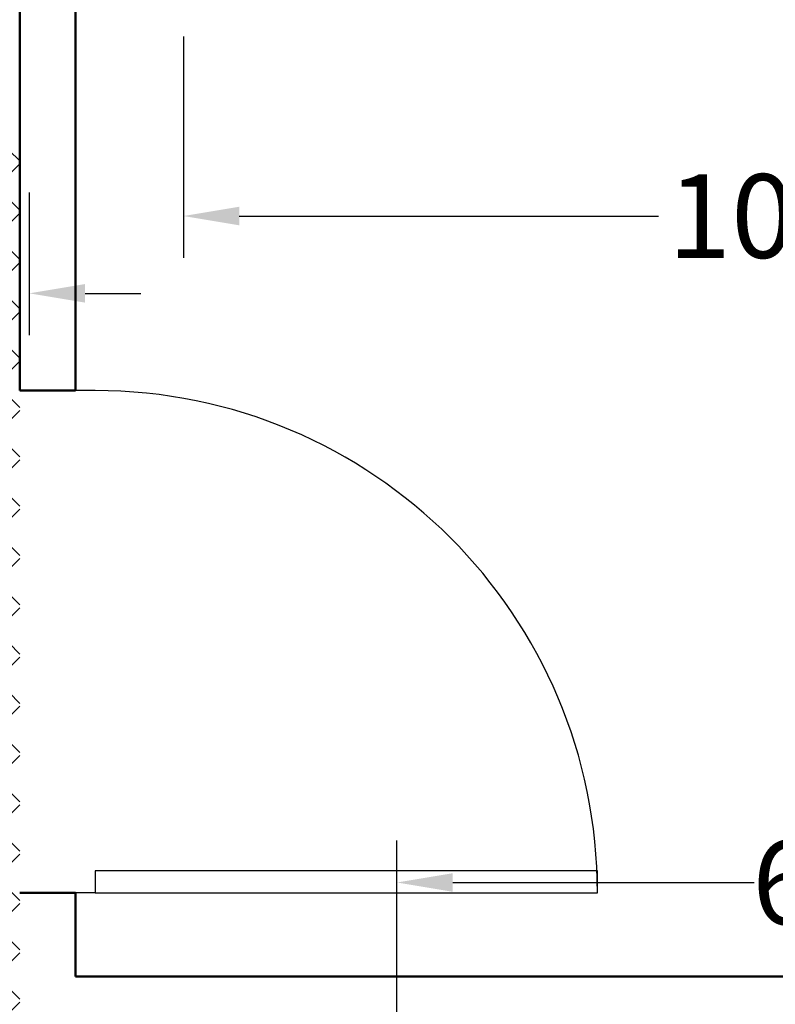
# Model space of a CAD drawing. Units: inches. Extents: x -466983 to 1020, y 324 to 318697.
# Tile 93 of 97: x 810 to 864, y 827 to 898. Entities that reach past the tile are written whole.
import ezdxf

# ---------------------------------------------------------------- set-up
doc = ezdxf.new("R2010")
doc.units = ezdxf.units.IN
doc.header["$MEASUREMENT"] = 0
for name, color, linetype, lineweight in [('A-ANNO-DIMS', 2, 'Continuous', 18), ('A-DOOR', 3, 'Continuous', 25), ('A-FLOR-PATT', 252, 'Continuous', 13), ('A-FURN', 8, 'Continuous', 18), ('A-WALL', 7, 'Continuous', 50)]:
    doc.layers.add(name, color=color, linetype=linetype, lineweight=lineweight)
doc.styles.get("Standard").update_dxf_attribs({"font": 'arial.ttf'})
doc.dimstyles.get("Standard").update_dxf_attribs({"dimtxt": 6, "dimasz": 4, "dimexe": 3, "dimexo": 3, "dimgap": 0.09, "dimtad": 0, "dimtih": 1, "dimtoh": 1, "dimdec": 1, "dimzin": 0, "dimdsep": 46, "dimlunit": 3, "dimtxsty": 'Standard', "dimcen": 0.09, "dimadec": 0, "dimazin": 0, "dimtfac": 1, "dimtdec": 1, "dimtofl": 0, "dimtmove": 0, "dimatfit": 3, "dimfxl": 1, "dimtolj": 1, "dimtzin": 0, "dimarcsym": 0})

# ---------------------------------------------------------------- blocks, each defined once
blk = doc.blocks.new('*U36')
for p, q in [((0, 0), (0, 6)), ((40, 0), (40, 6))]:
    blk.add_line(p, q)
blk.add_lwpolyline([(0, 0), (0, -40), (1.75, -40), (1.75, 0)], close=True)
blk.add_arc((0, 0), 40, 270, 0)
blk = doc.blocks.new('L Shaped Sofa')
at = {"ltscale": 2}
blk.add_arc((2416.36, 1205.03), 481.82, 262.8867, 276.632, dxfattribs=at)
blk = doc.blocks.new('*D71')
at = {"layer": 'A-ANNO-DIMS', "color": 0, "lineweight": -2, "transparency": 16777216}
for p, q in [((742.215, 885.152), (742.215, 874.91)), ((810.492, 885.152), (810.492, 874.91)), ((738.215, 877.91), (734.215, 877.91)), ((814.492, 877.91), (818.492, 877.91))]:
    blk.add_line(p, q, dxfattribs=at)
at = {"layer": 'A-ANNO-DIMS', "color": 0, "transparency": 16777216}
for points in [[(738.215, 878.577), (738.215, 877.244), (742.215, 877.91)], [(814.492, 878.577), (814.492, 877.244), (810.492, 877.91)]]:
    blk.add_solid(points, dxfattribs=at)
at = {"layer": 'Defpoints', "color": 0, "transparency": 16777216}
for p in [(742.215, 888.152), (810.492, 888.152), (742.215, 877.91)]:
    blk.add_point(p, dxfattribs=at)
at = {"layer": 'A-ANNO-DIMS', "color": 0, "transparency": 16777216, "insert": (776.354, 877.91), "char_height": 6, "attachment_point": 5}
blk.add_mtext('\\A1;L-SOFA 68 TYP.', dxfattribs=at)
blk = doc.blocks.new('*D74')
at = {"layer": 'A-ANNO-DIMS', "color": 0, "lineweight": -2, "transparency": 16777216}
for p, q in [((821.534, 896.315), (821.534, 880.453)), ((923.134, 896.315), (923.134, 880.453)), ((825.534, 883.453), (855.592, 883.453)), ((919.134, 883.453), (889.075, 883.453))]:
    blk.add_line(p, q, dxfattribs=at)
at = {"layer": 'A-ANNO-DIMS', "color": 0, "transparency": 16777216}
for points in [[(825.534, 884.119), (825.534, 882.786), (821.534, 883.453)], [(919.134, 884.119), (919.134, 882.786), (923.134, 883.453)]]:
    blk.add_solid(points, dxfattribs=at)
at = {"layer": 'Defpoints', "color": 0, "transparency": 16777216}
for p in [(821.534, 899.315), (923.134, 899.315), (923.134, 883.453)]:
    blk.add_point(p, dxfattribs=at)
at = {"layer": 'A-ANNO-DIMS', "color": 0, "transparency": 16777216, "insert": (872.334, 883.453), "char_height": 6, "attachment_point": 5}
blk.add_mtext('\\A1;102 TYP.', dxfattribs=at)
blk = doc.blocks.new('*D100')
at = {"layer": 'A-ANNO-DIMS', "color": 0, "lineweight": -2, "transparency": 16777216}
for p, q in [((836.84, 825.679), (836.84, 838.67)), ((896.84, 825.679), (896.84, 838.67)), ((840.84, 835.67), (862.447, 835.67)), ((892.84, 835.67), (871.234, 835.67))]:
    blk.add_line(p, q, dxfattribs=at)
at = {"layer": 'A-ANNO-DIMS', "color": 0, "transparency": 16777216}
for points in [[(840.84, 836.336), (840.84, 835.003), (836.84, 835.67)], [(892.84, 836.336), (892.84, 835.003), (896.84, 835.67)]]:
    blk.add_solid(points, dxfattribs=at)
at = {"layer": 'Defpoints', "color": 0, "transparency": 16777216}
for p in [(896.84, 835.67), (836.84, 822.679), (896.84, 822.679)]:
    blk.add_point(p, dxfattribs=at)
at = {"layer": 'A-ANNO-DIMS', "color": 0, "transparency": 16777216, "insert": (866.84, 835.67), "char_height": 6, "attachment_point": 5}
blk.add_mtext('\\A1;60', dxfattribs=at)

msp = doc.modelspace()

# ---------------------------------------------------------------- hatches: boundary and pattern name
at = {"layer": 'A-FLOR-PATT', "transparency": 33554572}
h = msp.add_hatch(dxfattribs=at)
h.set_pattern_fill('ANSI37', color=256, scale=30)
h.set_pattern_definition([(45, (-1212.4137, -290.035), (-2.6516504, 2.6516504), []), (135, (-1212.4137, -290.035), (-2.6516504, -2.6516504), [])])
h.paths.add_polyline_path([(901.806, 1075.938), (900.614, 1075.938), (900.614, 1065.386), (899.391, 1065.386), (898.091, 1065.386), (892.836, 1058.71, -0.258377), (892.188, 1058.351), (879.985, 1058.351, -0.20177), (879.438, 1058.581), (874.081, 1065.386), (872.781, 1065.386), (871.558, 1065.386), (871.558, 1075.938), (813.806, 1075.938), (813.806, 1044.792), (832.395, 1044.792, -0.394795), (848.66, 1028.536), (848.66, 1009.938), (901.806, 1009.938), (901.806, 1015.938), (901.306, 1015.938), (871.306, 1015.938), (871.306, 1017.25), (871.334, 1017.25, -0.401453), (901.306, 1045.938), (901.806, 1045.938)])
edge = h.paths.add_edge_path(flags=16)
edge.add_line((847.773, 1068.949), (847.773, 1073.709))
edge.add_arc((849.227, 1073.709), 1.454, 90, 180, ccw=False)
edge.add_line((849.227, 1075.163), (864.492, 1075.163))
edge.add_arc((864.492, 1073.709), 1.454, 0, 90, ccw=False)
edge.add_line((865.946, 1073.709), (865.946, 1069.004))
edge.add_arc((832.645, 1068.976), 33.301, -20.61234, 0.04725, ccw=False)
edge.add_ellipse((856.859, 1058.48), major_axis=(0, 10.213), ratio=0.685919, start_angle=100.00884, end_angle=259.99116, ccw=False)
edge.add_arc((881.074, 1068.976), 33.301, 180.04725, 200.61234, ccw=False)
h.paths.add_polyline_path([(853.146, 1066.482), (853.146, 1066.453), (853.146, 1066.453, 0.433107), (852.917, 1066.685), (852.917, 1066.453), (853.146, 1066.453), (853.146, 1066.482), (853.088, 1066.612, 0.697939), (852.7, 1066.453), (852.7, 1066.453), (852.7, 1066.482), (852.917, 1067.001), (852.917, 1066.685, -0.396254)], flags=0)
h.paths.add_polyline_path([(861.019, 1066.482), (861.019, 1066.453), (861.019, 1066.453, 0.416404), (860.802, 1066.685), (860.802, 1066.453), (861.019, 1066.453), (861.019, 1066.482), (860.967, 1066.605, 0.713344), (860.573, 1066.453), (860.573, 1066.453), (860.573, 1066.482), (860.802, 1067.001), (860.802, 1066.685, -0.379973)], flags=0)
edge = h.paths.add_edge_path(flags=0)
edge.add_spline(control_points=[(861.13, 1065.785), (861.466, 1065.248), (861.613, 1065.016), (861.983, 1064.374), (862.192, 1063.944), (862.561, 1063.039), (862.721, 1062.563), (862.987, 1061.578), (863.092, 1061.069), (863.245, 1060.031), (863.293, 1059.503), (863.329, 1058.441), (863.318, 1057.908), (863.237, 1056.852), (863.166, 1056.329), (862.97, 1055.308), (862.843, 1054.81), (862.537, 1053.852), (862.357, 1053.393), (861.951, 1052.525), (861.725, 1052.117), (861.233, 1051.362), (860.967, 1051.016), (860.405, 1050.395), (860.108, 1050.12), (859.494, 1049.646), (859.176, 1049.448), (858.528, 1049.13), (858.197, 1049.011), (857.531, 1048.852), (857.196, 1048.812), (856.525, 1048.812), (856.189, 1048.852), (855.524, 1049.01), (855.193, 1049.129), (854.545, 1049.447), (854.227, 1049.645), (853.612, 1050.118), (853.316, 1050.393), (852.753, 1051.014), (852.487, 1051.36), (851.995, 1052.114), (851.769, 1052.523), (851.363, 1053.39), (851.183, 1053.85), (850.877, 1054.807), (850.75, 1055.305), (850.553, 1056.326), (850.483, 1056.849), (850.401, 1057.905), (850.39, 1058.438), (850.426, 1059.5), (850.473, 1060.028), (850.626, 1061.066), (850.732, 1061.575), (850.997, 1062.561), (851.157, 1063.036), (851.525, 1063.942), (851.734, 1064.371), (852.106, 1065.016), (852.254, 1065.25), (852.608, 1065.733)], knot_values=[3.915332, 3.915332, 3.915332, 3.915332, 4.013468, 4.013468, 4.175532, 4.175532, 4.337596, 4.337596, 4.49966, 4.49966, 4.661724, 4.661724, 4.823788, 4.823788, 4.985852, 4.985852, 5.147916, 5.147916, 5.30998, 5.30998, 5.472044, 5.472044, 5.634109, 5.634109, 5.796173, 5.796173, 5.958237, 5.958237, 6.120301, 6.120301, 6.282365, 6.282365, 6.444429, 6.444429, 6.606493, 6.606493, 6.768557, 6.768557, 6.930621, 6.930621, 7.092685, 7.092685, 7.254749, 7.254749, 7.416813, 7.416813, 7.578878, 7.578878, 7.740942, 7.740942, 7.903006, 7.903006, 8.06507, 8.06507, 8.227134, 8.227134, 8.389198, 8.389198, 8.551262, 8.551262, 8.65037, 8.65037, 8.65037, 8.65037], degree=3, periodic=0)
edge.add_line((852.642, 1065.785), (861.13, 1065.785))
edge = h.paths.add_edge_path(flags=0)
edge.add_ellipse((856.85, 1057.743), major_axis=(0, 7.792), ratio=0.687861, start_angle=0, end_angle=360)
h.paths.add_polyline_path([(848.863, 1069.389), (848.863, 1073.96, -0.414214), (849.954, 1075.051), (863.765, 1075.051, -0.414214), (864.856, 1073.96), (864.856, 1069.389, -0.388936), (864.524, 1069.027, -0.043561), (849.195, 1069.027, -0.388936)], flags=0)
h.paths.add_polyline_path([(853.101, 1068.112, -1), (852.677, 1068.112, -1)], flags=0)
edge = h.paths.add_edge_path(flags=0)
edge.add_ellipse((856.859, 1057.338), major_axis=(0, 2.207), ratio=0.657164, start_angle=0, end_angle=360)
h.paths.add_polyline_path([(861.041, 1068.112, -1), (860.618, 1068.112, -1)], flags=0)
edge = h.paths.add_edge_path()
edge.add_line((573.954, 1057.341), (573.954, 1075.938))
edge.add_line((573.954, 1075.938), (558.731, 1075.938))
edge.add_line((558.731, 1075.938), (558.731, 1065.386))
edge.add_line((558.731, 1065.386), (557.507, 1065.386))
edge.add_line((557.507, 1065.386), (556.207, 1065.386))
edge.add_line((556.207, 1065.386), (550.952, 1058.71))
edge.add_arc((550.304, 1059.116), 0.765, 270, 327.94832, ccw=False)
edge.add_line((550.304, 1058.351), (538.101, 1058.351))
edge.add_arc((538.101, 1059.116), 0.765, 224.3704, 270, ccw=False)
edge.add_line((537.555, 1058.581), (532.198, 1065.386))
edge.add_line((532.198, 1065.386), (530.898, 1065.386))
edge.add_line((530.898, 1065.386), (529.674, 1065.386))
edge.add_line((529.674, 1065.386), (529.674, 1075.938))
edge.add_line((529.674, 1075.938), (520.806, 1075.938))
edge.add_line((520.806, 1075.938), (520.806, 1045.938))
edge.add_line((520.806, 1045.938), (521.306, 1045.938))
edge.add_arc((521.306, 1015.938), 30, 2.50749, 90, ccw=False)
edge.add_line((551.277, 1017.25), (551.306, 1017.25))
edge.add_line((551.306, 1017.25), (551.306, 1015.938))
edge.add_line((551.306, 1015.938), (520.806, 1015.938))
edge.add_line((520.806, 1015.938), (520.806, 1009.938))
edge.add_line((520.806, 1009.938), (559.191, 1010.402))
edge.add_arc((559.191, 1011.856), 1.454, 180, 270, ccw=False)
edge.add_line((557.737, 1011.856), (557.737, 1016.561))
edge.add_arc((591.039, 1016.589), 33.301, 159.38766, 180.04725, ccw=False)
edge.add_ellipse((566.824, 1027.085), major_axis=(0, 10.213), ratio=0.685919, start_angle=280.00884, end_angle=439.99116, ccw=False)
edge.add_arc((542.609, 1016.589), 33.301, 0.04725, 20.61234, ccw=False)
edge.add_line((575.91, 1016.616), (575.91, 1011.856))
edge.add_arc((574.456, 1011.856), 1.454, -90, 0, ccw=False)
edge.add_line((574.456, 1010.402), (608.806, 1009.938))
edge.add_line((608.806, 1009.938), (608.806, 1041.086))
edge.add_line((608.806, 1041.086), (590.218, 1041.086))
edge.add_arc((590.775, 1057.907), 16.831, 181.92775, 268.10321, ccw=False)
edge = h.paths.add_edge_path()
edge.add_ellipse((494.244, 583.62), major_axis=(0, 10.213), ratio=0.685919, start_angle=280.00884, end_angle=439.99116, ccw=False)
edge.add_arc((470.03, 573.124), 33.301, 0.04725, 20.61234, ccw=False)
edge.add_line((503.331, 573.152), (503.331, 568.392))
edge.add_arc((501.877, 568.392), 1.454, -90, 0, ccw=False)
edge.add_line((501.877, 566.938), (539.806, 566.938))
edge.add_line((539.806, 566.938), (539.806, 572.938))
edge.add_line((539.806, 572.938), (539.306, 572.938))
edge.add_line((539.306, 572.938), (509.306, 572.938))
edge.add_line((509.306, 572.938), (509.306, 574.25))
edge.add_line((509.306, 574.25), (509.334, 574.25))
edge.add_arc((539.306, 572.938), 30, 90, 177.49251, ccw=False)
edge.add_line((539.306, 602.938), (539.806, 602.938))
edge.add_line((539.806, 602.938), (539.806, 626.938))
edge.add_line((539.806, 626.938), (531.772, 626.938))
edge.add_line((531.772, 626.938), (531.772, 616.386))
edge.add_line((531.772, 616.386), (530.548, 616.386))
edge.add_line((530.548, 616.386), (529.249, 616.386))
edge.add_line((529.249, 616.386), (523.711, 609.351))
edge.add_line((523.711, 609.351), (510.777, 609.351))
edge.add_line((510.777, 609.351), (505.239, 616.386))
edge.add_line((505.239, 616.386), (503.939, 616.386))
edge.add_line((503.939, 616.386), (502.715, 616.386))
edge.add_line((502.715, 616.386), (502.715, 626.938))
edge.add_line((502.715, 626.938), (481.698, 626.938))
edge.add_line((481.698, 626.938), (481.698, 610.995))
edge.add_arc((467.27, 611.473), 14.436, 271.92775, 358.10321, ccw=False)
edge.add_line((467.756, 597.045), (451.806, 597.045))
edge.add_line((451.806, 597.045), (451.806, 584.404))
edge.add_line((451.806, 584.404), (451.806, 566.938))
edge.add_line((451.806, 566.938), (486.612, 566.938))
edge.add_arc((486.612, 568.392), 1.454, 180, 270, ccw=False)
edge.add_line((485.158, 568.392), (485.158, 573.097))
edge.add_arc((518.459, 573.124), 33.301, 159.38766, 180.04725, ccw=False)
h.paths.add_polyline_path([(836.261, 1020.733), (879.89, 1020.733), (879.89, 1039.39), (836.261, 1039.39)], flags=25)
h.paths.add_polyline_path([(549.985, 1036.749), (593.614, 1036.749), (593.614, 1055.407), (549.985, 1055.407)], flags=24)
h.paths.add_polyline_path([(475.123, 595.596), (518.752, 595.596), (518.752, 614.253), (475.123, 614.253)], flags=24)
h = msp.add_hatch(dxfattribs=at)
h.set_pattern_fill('ANSI37', color=256, scale=20)
h.set_pattern_definition([(45, (-1212.4137, -290.035), (-1.767767, 1.767767), []), (135, (-1212.4137, -290.035), (-1.767767, -1.767767), [])])
h.paths.add_polyline_path([(809.806, 870.938), (809.806, 888.152), (806.998, 888.152), (802.662, 888.152), (789.383, 888.152), (786.285, 888.152, -0.414214), (785.499, 888.937), (785.499, 900.196), (785.499, 908.47, -0.414214), (786.808, 909.779, -0.414214), (785.499, 911.088), (785.499, 929.101, -0.414214), (786.808, 930.411, -0.414214), (785.499, 931.72), (785.499, 931.904, -0.414214), (784.19, 930.595), (766.722, 930.595, -0.412359), (765.413, 931.896, -0.413741), (764.115, 930.578), (744.578, 930.422, -0.416556), (743.786, 931.207), (743.786, 933.515), (742.215, 933.515), (742.215, 952.024, -0.001344), (743.786, 952.2), (743.786, 953.938), (678.592, 953.938), (678.592, 951.131), (678.592, 946.794), (678.592, 933.515), (678.592, 930.417, -0.414214), (677.806, 929.631), (666.548, 929.631), (658.274, 929.631, -0.414214), (656.965, 930.94, -0.414214), (655.656, 929.631), (637.642, 929.631, -0.414214), (636.333, 930.94, -0.414214), (635.024, 929.631), (634.839, 929.631, -0.414214), (636.149, 928.322), (636.149, 910.854, -0.412359), (634.848, 909.545, -0.413741), (636.165, 908.247), (636.321, 888.71, -0.416556), (635.536, 887.918), (633.228, 887.918), (633.228, 886.347), (614.719, 886.347, -0.001344), (614.544, 887.918), (612.806, 887.918), (612.806, 834.938), (612.806, 752.938), (612.806, 748.938), (612.806, 697.938), (654.806, 697.938), (654.806, 701.938), (715.806, 701.938), (715.806, 737.435), (774.292, 737.435), (774.292, 795.938), (809.806, 795.938)])
h.paths.add_polyline_path([(679.276, 849.576, 0.102523), (682.148, 849.261, -0.080461), (694.543, 849.773, -0.283899), (694.482, 849.008, 0.136605), (694.407, 848.81, -0.030441), (694.543, 846.893), (694.543, 842.62), (694.543, 838.347, -0.028219), (694.425, 836.568), (694.425, 836.568, 0.196187), (694.446, 836.271, -0.302897), (694.543, 835.467, -0.080461), (682.148, 835.979, 0.102523), (679.276, 835.664, -0.58611), (678.646, 836.017), (678.646, 849.223, -0.58611)], flags=16)
h.paths.add_polyline_path([(679.517, 848.651, 0.699597), (679.476, 848.634, 1.20716), (679.194, 848.742, 0.010621)], flags=0)
h.paths.add_polyline_path([(679.492, 836.561, -0.013798), (679.918, 836.659, -0.071703), (682.853, 837.143, -0.165743), (682.166, 839.101), (682.166, 842.609), (682.166, 846.06, -0.240616), (683.473, 848.677, -0.068263), (693.929, 849.008), (693.788, 848.708), (693.788, 849.023, 0.067332), (683.473, 848.677, 0.240616), (682.166, 846.06), (682.166, 842.609), (682.166, 839.101, 0.23459), (683.461, 836.551, 0.068093), (693.788, 836.195), (693.788, 836.51), (693.93, 836.21, -0.077215), (682.242, 836.782, 0.086627), (679.528, 836.57, -0.628402), (679.503, 836.573), (679.503, 836.607, 0.910458)], flags=0)
h.paths.add_polyline_path([(679.476, 848.636), (679.207, 848.647), (679.207, 836.572, 0.913566), (679.365, 836.586), (679.476, 836.582)], flags=0)
h.paths.add_polyline_path([(679.276, 829.86, 0.102523), (682.148, 829.546, -0.080461), (694.543, 830.057, -0.283899), (694.482, 829.293, 0.136605), (694.407, 829.095, -0.030441), (694.543, 827.178), (694.543, 822.904), (694.543, 818.631, -0.028219), (694.425, 816.853), (694.425, 816.853, 0.196187), (694.446, 816.556, -0.302897), (694.543, 815.752, -0.080461), (682.148, 816.263, 0.102523), (679.276, 815.949, -0.58611), (678.646, 816.302), (678.646, 829.507, -0.58611)], flags=16)
h.paths.add_polyline_path([(679.517, 828.936, 0.699597), (679.476, 828.919, 1.20716), (679.194, 829.027, 0.010621)], flags=0)
h.paths.add_polyline_path([(679.492, 816.846, -0.013798), (679.918, 816.944, -0.071703), (682.853, 817.428, -0.165743), (682.166, 819.385), (682.166, 822.894), (682.166, 826.345, -0.240616), (683.473, 828.961, -0.068263), (693.929, 829.293), (693.788, 828.993), (693.788, 829.308, 0.067332), (683.473, 828.961, 0.240616), (682.166, 826.345), (682.166, 822.894), (682.166, 819.385, 0.23459), (683.461, 816.836, 0.068093), (693.788, 816.48), (693.788, 816.795), (693.93, 816.495, -0.077215), (682.242, 817.066, 0.086627), (679.528, 816.855, -0.628402), (679.503, 816.858), (679.503, 816.892, 0.910458)], flags=0)
h.paths.add_polyline_path([(679.476, 828.921), (679.207, 828.932), (679.207, 816.857, 0.913566), (679.365, 816.871), (679.476, 816.867)], flags=0)
h.paths.add_polyline_path([(679.276, 810.145, 0.102523), (682.148, 809.83, -0.080461), (694.543, 810.342, -0.3023), (694.447, 809.539, 0.10023), (694.406, 809.388, -0.03057), (694.543, 807.462), (694.543, 803.189), (694.543, 798.916, -0.03057), (694.406, 796.991, 0.10023), (694.447, 796.839, -0.3023), (694.543, 796.036, -0.080461), (682.148, 796.548, 0.102523), (679.276, 796.233, -0.58611), (678.646, 796.586), (678.646, 809.792, -0.58611)], flags=16)
h.paths.add_polyline_path([(679.517, 809.242, 0.699597), (679.476, 809.224, 1.20716), (679.194, 809.332, 0.010621)], flags=0)
h.paths.add_polyline_path([(679.492, 797.151, -0.013798), (679.918, 797.25, -0.071703), (682.853, 797.734, -0.165743), (682.166, 799.691), (682.166, 803.2), (682.166, 806.65, -0.239349), (683.461, 809.258, -0.072465), (694.447, 809.541, 0.197932), (694.425, 809.241), (693.788, 809.299), (693.788, 809.614, 0.068093), (683.461, 809.258, 0.239349), (682.166, 806.65), (682.166, 803.2), (682.166, 799.691, 0.235854), (683.473, 797.132, 0.067332), (693.788, 796.786), (693.788, 797.101), (694.425, 797.159, 0.197932), (694.447, 796.859, -0.080419), (682.156, 797.379, 0.083867), (679.528, 797.16, -0.628402), (679.503, 797.164), (679.503, 797.197, 0.910458)], flags=0)
h.paths.add_polyline_path([(679.207, 809.237), (679.207, 797.162, 0.913566), (679.365, 797.176), (679.476, 797.173), (679.476, 809.227)], flags=0)
h.paths.add_polyline_path([(695.364, 853.299), (728.223, 853.299), (728.223, 771.152), (695.364, 771.152)], flags=16)
h.paths.add_polyline_path([(696.021, 852.642), (727.566, 852.642), (727.566, 771.809), (696.021, 771.809)], flags=0)
h.paths.add_polyline_path([(679.276, 788.787, 0.102523), (682.148, 788.472, -0.080461), (694.543, 788.984, -0.3023), (694.447, 788.181, 0.10023), (694.406, 788.03, -0.03057), (694.543, 786.104), (694.543, 781.831), (694.543, 777.558, -0.03057), (694.406, 775.632, 0.10023), (694.447, 775.481, -0.3023), (694.543, 774.678, -0.080461), (682.148, 775.19, 0.102523), (679.276, 774.875, -0.58611), (678.646, 775.228), (678.646, 788.434, -0.58611)], flags=16)
h.paths.add_polyline_path([(679.517, 787.883, 0.699597), (679.476, 787.866, 1.20716), (679.194, 787.974, 0.010621)], flags=0)
h.paths.add_polyline_path([(679.492, 775.793, -0.013798), (679.918, 775.891, -0.071703), (682.853, 776.375, -0.165743), (682.166, 778.333), (682.166, 781.841), (682.166, 785.292, -0.239349), (683.461, 787.899, -0.072465), (694.447, 788.182, 0.197932), (694.425, 787.882), (693.788, 787.94), (693.788, 788.255, 0.068093), (683.461, 787.899, 0.239349), (682.166, 785.292), (682.166, 781.841), (682.166, 778.333, 0.235854), (683.473, 775.774, 0.067332), (693.788, 775.428), (693.788, 775.742), (694.425, 775.8, 0.197932), (694.447, 775.5, -0.080419), (682.156, 776.021, 0.083867), (679.528, 775.802, -0.628402), (679.503, 775.805), (679.503, 775.839, 0.910458)], flags=0)
h.paths.add_polyline_path([(679.207, 787.879), (679.207, 775.804, 0.913566), (679.365, 775.818), (679.476, 775.814), (679.476, 787.868)], flags=0)
h.paths.add_polyline_path([(704.641, 854.12, -0.080461), (705.153, 866.516, 0.102523), (704.838, 869.387, -0.58611), (705.191, 870.017), (718.397, 870.017, -0.58611), (718.75, 869.387, 0.102523), (718.435, 866.516, -0.080461), (718.946, 854.12, -0.3023), (718.144, 854.217, 0.10023), (717.992, 854.257, -0.03057), (716.067, 854.12), (711.794, 854.12), (707.521, 854.12, -0.03057), (705.595, 854.257, 0.10023), (705.444, 854.217, -0.3023)], flags=16)
h.paths.add_polyline_path([(717.846, 869.146, 0.699597), (717.829, 869.187, 1.20716), (717.937, 869.47, 0.010621)], flags=0)
h.paths.add_polyline_path([(705.463, 854.216, -0.080419), (705.984, 866.507, 0.083867), (705.765, 869.135, -0.628402), (705.768, 869.16), (705.802, 869.16, 0.910458), (705.756, 869.171, -0.013798), (705.854, 868.745, -0.071703), (706.338, 865.81, -0.165743), (708.295, 866.497), (711.804, 866.497), (715.255, 866.497, -0.239349), (717.862, 865.202, -0.072465), (718.145, 854.216, 0.197932), (717.845, 854.238), (717.903, 854.876), (718.218, 854.876, 0.068093), (717.862, 865.202, 0.239349), (715.255, 866.497), (711.804, 866.497), (708.295, 866.497, 0.235854), (705.737, 865.19, 0.067332), (705.391, 854.876), (705.705, 854.876), (705.763, 854.238, 0.197932)], flags=16)
h.paths.add_polyline_path([(705.766, 869.456, 0.913566), (705.781, 869.299), (705.777, 869.187), (717.831, 869.187), (717.842, 869.456)], flags=0)
h.paths.add_polyline_path([(729.045, 842.62), (729.045, 846.893, -0.03057), (729.182, 848.818, 0.10023), (729.141, 848.97, -0.3023), (729.045, 849.773, -0.080461), (741.44, 849.261, 0.102523), (744.311, 849.576, -0.58611), (744.942, 849.223), (744.942, 836.017, -0.58611), (744.311, 835.664, 0.102523), (741.44, 835.979, -0.080461), (729.045, 835.467, -0.3023), (729.141, 836.27, 0.10023), (729.182, 836.421, -0.03057), (729.045, 838.347)], flags=16)
h.paths.add_polyline_path([(744.111, 836.585, 1.20716), (744.394, 836.477, 0.010621), (744.07, 836.567, 0.699597)], flags=0)
h.paths.add_polyline_path([(729.141, 836.268, 0.197932), (729.162, 836.568), (729.8, 836.51), (729.8, 836.195, 0.068093), (740.126, 836.551, 0.239349), (741.421, 839.159), (741.421, 842.609), (741.421, 846.118, 0.235854), (740.114, 848.677, 0.067332), (729.8, 849.023), (729.8, 848.708), (729.162, 848.65, 0.197932), (729.141, 848.95, -0.080419), (741.432, 848.43, 0.083867), (744.059, 848.649, -0.628402), (744.085, 848.645), (744.085, 848.612, 0.910458), (744.095, 848.658, -0.013798), (743.67, 848.559, -0.071703), (740.734, 848.075, -0.165743), (741.421, 846.118), (741.421, 842.609), (741.421, 839.159, -0.239349), (740.126, 836.551, -0.072465)], flags=0)
h.paths.add_polyline_path([(729.045, 830.057, -0.080461), (741.44, 829.546, 0.102523), (744.311, 829.86, -0.58611), (744.942, 829.507), (744.942, 816.302, -0.58611), (744.311, 815.949, 0.102523), (741.44, 816.263, -0.080461), (729.045, 815.752, -0.3023), (729.141, 816.554, 0.10023), (729.182, 816.706, -0.03057), (729.045, 818.631), (729.045, 822.904), (729.045, 827.178, -0.03057), (729.182, 829.103, 0.10023), (729.141, 829.255, -0.3023)], flags=16)
h.paths.add_polyline_path([(744.111, 816.869, 1.20716), (744.394, 816.761, 0.010621), (744.07, 816.852, 0.699597)], flags=0)
h.paths.add_polyline_path([(729.141, 829.235, -0.080419), (741.432, 828.714, 0.083867), (744.059, 828.933, -0.628402), (744.085, 828.93), (744.085, 828.896, 0.910458), (744.095, 828.943, -0.013798), (743.67, 828.844, -0.071703), (740.734, 828.36, -0.165743), (741.421, 826.403), (741.421, 822.894), (741.421, 819.443, -0.239349), (740.126, 816.836, -0.072465), (729.141, 816.553, 0.197932), (729.162, 816.853), (729.8, 816.795), (729.8, 816.48, 0.068093), (740.126, 816.836, 0.239349), (741.421, 819.443), (741.421, 822.894), (741.421, 826.403, 0.235854), (740.114, 828.961, 0.067332), (729.8, 829.308), (729.8, 828.993), (729.162, 828.935, 0.197932)], flags=16)
h.paths.add_polyline_path([(729.045, 810.342, -0.080461), (741.44, 809.83, 0.102523), (744.311, 810.145, -0.58611), (744.942, 809.792), (744.942, 796.586, -0.58611), (744.311, 796.233, 0.102523), (741.44, 796.548, -0.080461), (729.045, 796.036, -0.283899), (729.105, 796.801, 0.136605), (729.181, 796.999, -0.030441), (729.045, 798.916), (729.045, 803.189), (729.045, 807.462, -0.028219), (729.163, 809.241), (729.162, 809.241, 0.196187), (729.142, 809.538, -0.302897)], flags=16)
h.paths.add_polyline_path([(744.111, 797.175, 1.20716), (744.394, 797.067, 0.010621), (744.07, 797.158, 0.699597)], flags=0)
h.paths.add_polyline_path([(741.345, 809.027, 0.086627), (744.059, 809.239, -0.628402), (744.085, 809.235), (744.085, 809.202, 0.910458), (744.095, 809.248, -0.013798), (743.67, 809.15, -0.071703), (740.734, 808.666, -0.165743), (741.421, 806.708), (741.421, 803.2), (741.421, 799.749, -0.240616), (740.114, 797.132, -0.068263), (729.658, 796.801), (729.8, 797.101), (729.8, 796.786, 0.067332), (740.114, 797.132, 0.240616), (741.421, 799.749), (741.421, 803.2), (741.421, 806.708, 0.23459), (740.126, 809.258, 0.068093), (729.8, 809.614), (729.8, 809.299), (729.658, 809.599, -0.077215)], flags=0)
h.paths.add_polyline_path([(704.641, 770.33, -0.283899), (705.405, 770.27, 0.136605), (705.603, 770.194, -0.030441), (707.521, 770.33), (711.794, 770.33), (716.067, 770.33, -0.028219), (717.845, 770.212), (717.845, 770.213, 0.196187), (718.143, 770.233, -0.302897), (718.946, 770.33, -0.080461), (718.435, 757.935, 0.102523), (718.75, 755.064, -0.58611), (718.397, 754.433), (705.191, 754.433, -0.58611), (704.838, 755.064, 0.102523), (705.153, 757.935, -0.080461)], flags=16)
h.paths.add_polyline_path([(705.762, 755.305, 0.699597), (705.779, 755.264, 1.20716), (705.671, 754.981, 0.010621)], flags=0)
h.paths.add_polyline_path([(705.405, 769.717), (705.705, 769.575), (705.391, 769.575, 0.067332), (705.737, 759.261, 0.240616), (708.353, 757.954), (711.804, 757.954), (715.313, 757.954, 0.23459), (717.862, 759.249, 0.068093), (718.218, 769.575), (717.903, 769.575), (718.203, 769.717, -0.077215), (717.632, 758.03, 0.086627), (717.843, 755.316, -0.628402), (717.84, 755.29), (717.806, 755.29, 0.910458), (717.853, 755.28, -0.013798), (717.754, 755.705, -0.071703), (717.27, 758.641, -0.165743), (715.313, 757.954), (711.804, 757.954), (708.353, 757.954, -0.240616), (705.737, 759.261, -0.068263)], flags=0)
h.paths.add_polyline_path([(729.045, 788.984, -0.080461), (741.44, 788.472, 0.102523), (744.311, 788.787, -0.58611), (744.942, 788.434), (744.942, 775.228, -0.58611), (744.311, 774.875, 0.102523), (741.44, 775.19, -0.080461), (729.045, 774.678, -0.283899), (729.105, 775.443, 0.136605), (729.181, 775.64, -0.030441), (729.045, 777.558), (729.045, 781.831), (729.045, 786.104, -0.028219), (729.163, 787.882), (729.162, 787.882, 0.196187), (729.142, 788.18, -0.302897)], flags=16)
h.paths.add_polyline_path([(744.111, 775.817, 1.20716), (744.394, 775.709, 0.010621), (744.07, 775.799, 0.699597)], flags=0)
h.paths.add_polyline_path([(741.345, 787.669, 0.086627), (744.059, 787.881, -0.628402), (744.085, 787.877), (744.085, 787.844, 0.910458), (744.095, 787.89, -0.013798), (743.67, 787.791, -0.071703), (740.734, 787.307, -0.165743), (741.421, 785.35), (741.421, 781.841), (741.421, 778.39, -0.240616), (740.114, 775.774, -0.068263), (729.658, 775.443), (729.8, 775.742), (729.8, 775.428, 0.067332), (740.114, 775.774, 0.240616), (741.421, 778.39), (741.421, 781.841), (741.421, 785.35, 0.23459), (740.126, 787.899, 0.068093), (729.8, 788.255), (729.8, 787.94), (729.658, 788.241, -0.077215)], flags=0)
h.paths.add_polyline_path([(744.111, 848.636), (744.111, 836.582), (744.381, 836.572), (744.381, 848.647, 0.913566), (744.223, 848.633)], flags=0)
h.paths.add_polyline_path([(744.223, 828.917), (744.111, 828.921), (744.111, 816.867), (744.381, 816.857), (744.381, 828.932, 0.913566)], flags=0)
h.paths.add_polyline_path([(717.831, 755.264), (705.777, 755.264), (705.766, 754.994), (717.842, 754.994, 0.913566), (717.827, 755.152)], flags=0)
h.paths.add_polyline_path([(744.223, 809.223), (744.111, 809.227), (744.111, 797.173), (744.381, 797.162), (744.381, 809.237, 0.913566)], flags=0)
h.paths.add_polyline_path([(744.111, 787.868), (744.111, 775.814), (744.381, 775.804), (744.381, 787.879, 0.913566), (744.223, 787.865)], flags=0)
h.paths.add_polyline_path([(678.877, 877.123), (737.613, 877.123), (737.613, 899.512), (678.877, 899.512)], flags=24)

# ---------------------------------------------------------------- linework, layer by layer
at = {"layer": 'A-WALL'}
for p, q in [((813.806, 1005.938), (813.806, 870.938)), ((809.806, 953.938), (809.806, 870.938)), ((813.806, 870.938), (809.806, 870.938)), ((813.806, 834.938), (809.806, 834.938)), ((813.806, 834.938), (813.806, 828.938)), ((982.806, 828.938), (813.806, 828.938))]:
    msp.add_line(p, q, dxfattribs=at)

# ---------------------------------------------------------------- block references
at = {"layer": 'A-DOOR', "xscale": 0.8999999999999942, "yscale": 0.8999999999999942, "zscale": 0.8999999999999942, "rotation": 90}
msp.add_blockref('*U36', (815.206, 834.938), dxfattribs=at)
at = {"layer": 'A-FURN', "xscale": 0.5482153745360612, "yscale": 0.5482153745360612, "zscale": 0.5482153745360612, "rotation": 89.99999999999999}
msp.add_blockref('L Shaped Sofa', (1206.291, -403.039), dxfattribs=at)

# ---------------------------------------------------------------- dimensions: what is measured, and where the dimension line sits
at = {"layer": 'A-ANNO-DIMS'}
dim = msp.add_linear_dim(base=(923.134, 883.453), p1=(821.534, 899.315), p2=(923.134, 899.315), text='<> TYP.', dimstyle='Standard', override={"dimdec": 0, "dimlfac": 1, "dimrnd": 0, "dimzin": 0, "dimdsep": 46, "dimlunit": 2}, dxfattribs=at)
dim.commit()
dim.dimension.update_dxf_attribs({"geometry": '*D74', "text_midpoint": (872.334, 883.453)})
dim = msp.add_linear_dim(base=(742.215, 877.91), p1=(810.492, 888.152), p2=(742.215, 888.152), angle=180, text='L-SOFA <> TYP.', dimstyle='Standard', override={"dimdec": 0, "dimlfac": 1, "dimrnd": 0, "dimzin": 0, "dimdsep": 46, "dimlunit": 2}, dxfattribs=at)
dim.commit()
dim.dimension.update_dxf_attribs({"geometry": '*D71', "text_midpoint": (776.354, 877.91)})
dim = msp.add_linear_dim(base=(896.84, 835.67), p1=(836.84, 822.679), p2=(896.84, 822.679), dimstyle='Standard', override={"dimdec": 0, "dimlfac": 1, "dimrnd": 0, "dimzin": 0, "dimdsep": 46, "dimlunit": 2}, dxfattribs=at)
dim.commit()
dim.dimension.update_dxf_attribs({"geometry": '*D100', "text_midpoint": (866.84, 835.67)})

doc.saveas('drawing.dxf')
